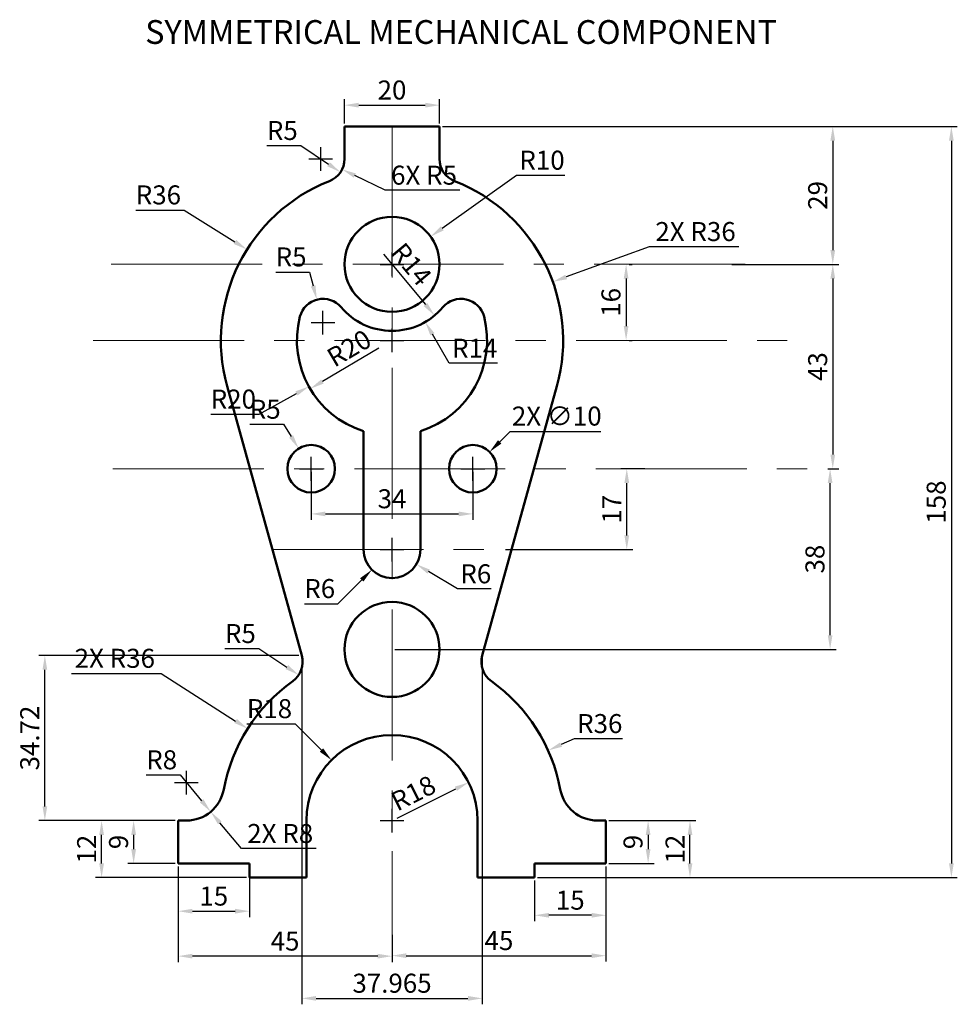
# Model space of a CAD drawing. Units: millimetres. Extents: x 53 to 250, y -7 to 201.
import ezdxf

# ---------------------------------------------------------------- set-up
doc = ezdxf.new("R2010")
doc.units = ezdxf.units.MM
doc.linetypes.add('CENTER', pattern=[50.8, 31.75, -6.35, 6.35, -6.35])
for name, color, linetype, lineweight in [('M-CNTR', 1, 'CENTER', 18), ('M-DIMS', 2, 'Continuous', 25), ('M-OUTL', 7, 'Continuous', 50), ('M-TEXT', 3, 'Continuous', 25)]:
    doc.layers.add(name, color=color, linetype=linetype, lineweight=lineweight)
doc.styles.get("Standard").update_dxf_attribs({"font": 'arial.ttf'})
doc.dimstyles.new('ISO-25', dxfattribs={"dimtxt": 4, "dimasz": 3, "dimexe": 1.25, "dimexo": 0.625, "dimtad": 1, "dimtoh": 1, "dimdec": 1, "dimtxsty": 'Standard', "dimcen": 2.5, "dimadec": 0, "dimazin": 0, "dimtfac": 1, "dimtdec": 1, "dimtofl": 0, "dimtmove": 0, "dimatfit": 3, "dimfxl": 1, "dimarcsym": 0})

# ---------------------------------------------------------------- blocks, each defined once
blk = doc.blocks.new('*D1')
at = {"layer": 'Defpoints', "color": 0, "transparency": 16777216}
for p in [(176.08, 32.09), (176.08, 23.09), (184.96, 23.09)]:
    blk.add_point(p, dxfattribs=at)
at = {"layer": 'M-DIMS', "color": 0, "lineweight": -2, "transparency": 16777216}
for p, q in [((176.7, 32.09), (186.21, 32.09)), ((184.96, 29.09), (184.96, 26.09)), ((176.7, 23.09), (186.21, 23.09))]:
    blk.add_line(p, q, dxfattribs=at)
at = {"layer": 'M-DIMS', "color": 0, "transparency": 16777216}
for points in [[(184.46, 29.09), (185.46, 29.09), (184.96, 32.09)], [(184.46, 26.09), (185.46, 26.09), (184.96, 23.09)]]:
    blk.add_solid(points, dxfattribs=at)
at = {"layer": 'M-DIMS', "color": 0, "transparency": 16777216, "insert": (182.3, 27.59), "char_height": 4, "attachment_point": 5, "rotation": 90}
blk.add_mtext('9', dxfattribs=at)
blk = doc.blocks.new('*D2')
at = {"layer": 'Defpoints', "color": 0, "transparency": 16777216}
for p in [(176.08, 32.09), (193.77, 32.09), (161.08, 20.09)]:
    blk.add_point(p, dxfattribs=at)
at = {"layer": 'M-DIMS', "color": 0, "lineweight": -2, "transparency": 16777216}
for p, q in [((176.7, 32.09), (195.02, 32.09)), ((193.77, 23.09), (193.77, 29.09)), ((161.7, 20.09), (195.02, 20.09))]:
    blk.add_line(p, q, dxfattribs=at)
at = {"layer": 'M-DIMS', "color": 0, "transparency": 16777216}
for points in [[(193.27, 29.09), (194.27, 29.09), (193.77, 32.09)], [(193.27, 23.09), (194.27, 23.09), (193.77, 20.09)]]:
    blk.add_solid(points, dxfattribs=at)
at = {"layer": 'M-DIMS', "color": 0, "transparency": 16777216, "insert": (191.14, 26.09), "char_height": 4, "attachment_point": 5, "rotation": 90}
blk.add_mtext('12', dxfattribs=at)
blk = doc.blocks.new('*D3')
at = {"layer": 'Defpoints', "color": 0, "transparency": 16777216}
for p in [(176.08, 23.09), (161.08, 20.09), (161.08, 12.18)]:
    blk.add_point(p, dxfattribs=at)
at = {"layer": 'M-DIMS', "color": 0, "lineweight": -2, "transparency": 16777216}
for p, q in [((176.08, 22.47), (176.08, 10.93)), ((161.08, 19.47), (161.08, 10.93)), ((173.08, 12.18), (164.08, 12.18))]:
    blk.add_line(p, q, dxfattribs=at)
at = {"layer": 'M-DIMS', "color": 0, "transparency": 16777216}
for points in [[(164.08, 12.68), (164.08, 11.68), (161.08, 12.18)], [(173.08, 12.68), (173.08, 11.68), (176.08, 12.18)]]:
    blk.add_solid(points, dxfattribs=at)
at = {"layer": 'M-DIMS', "color": 0, "transparency": 16777216, "insert": (168.58, 14.84), "char_height": 4, "attachment_point": 5}
blk.add_mtext('15', dxfattribs=at)
blk = doc.blocks.new('*D4')
at = {"layer": 'Defpoints', "color": 0, "transparency": 16777216}
for p in [(176.08, 23.09), (131.08, 7.05), (176.08, 3.68)]:
    blk.add_point(p, dxfattribs=at)
at = {"layer": 'M-DIMS', "color": 0, "lineweight": -2, "transparency": 16777216}
for p, q in [((176.08, 22.47), (176.08, 2.43)), ((131.08, 6.42), (131.08, 2.43)), ((134.08, 3.68), (173.08, 3.68))]:
    blk.add_line(p, q, dxfattribs=at)
at = {"layer": 'M-DIMS', "color": 0, "transparency": 16777216}
for points in [[(134.08, 4.18), (134.08, 3.18), (131.08, 3.68)], [(173.08, 4.18), (173.08, 3.18), (176.08, 3.68)]]:
    blk.add_solid(points, dxfattribs=at)
at = {"layer": 'M-DIMS', "color": 0, "transparency": 16777216, "insert": (153.58, 6.34), "char_height": 4, "attachment_point": 5}
blk.add_mtext('45', dxfattribs=at)
blk = doc.blocks.new('*D5')
at = {"layer": 'Defpoints', "color": 0, "transparency": 16777216}
for p in [(86.08, 23.09), (101.08, 23.09), (101.08, 13.04)]:
    blk.add_point(p, dxfattribs=at)
at = {"layer": 'M-DIMS', "color": 0, "lineweight": -2, "transparency": 16777216}
for p, q in [((86.08, 22.47), (86.08, 11.79)), ((101.08, 22.47), (101.08, 11.79)), ((89.08, 13.04), (98.08, 13.04))]:
    blk.add_line(p, q, dxfattribs=at)
at = {"layer": 'M-DIMS', "color": 0, "transparency": 16777216}
for points in [[(89.08, 13.54), (89.08, 12.54), (86.08, 13.04)], [(98.08, 13.54), (98.08, 12.54), (101.08, 13.04)]]:
    blk.add_solid(points, dxfattribs=at)
at = {"layer": 'M-DIMS', "color": 0, "transparency": 16777216, "insert": (93.58, 15.7), "char_height": 4, "attachment_point": 5}
blk.add_mtext('15', dxfattribs=at)
blk = doc.blocks.new('*D6')
at = {"layer": 'Defpoints', "color": 0, "transparency": 16777216}
for p in [(86.08, 32.09), (76.72, 23.09), (86.08, 23.09)]:
    blk.add_point(p, dxfattribs=at)
at = {"layer": 'M-DIMS', "color": 0, "lineweight": -2, "transparency": 16777216}
for p, q in [((85.45, 32.09), (75.47, 32.09)), ((76.72, 29.09), (76.72, 26.09)), ((85.45, 23.09), (75.47, 23.09))]:
    blk.add_line(p, q, dxfattribs=at)
at = {"layer": 'M-DIMS', "color": 0, "transparency": 16777216}
for points in [[(76.22, 29.09), (77.22, 29.09), (76.72, 32.09)], [(76.22, 26.09), (77.22, 26.09), (76.72, 23.09)]]:
    blk.add_solid(points, dxfattribs=at)
at = {"layer": 'M-DIMS', "color": 0, "transparency": 16777216, "insert": (74.06, 27.59), "char_height": 4, "attachment_point": 5, "rotation": 90}
blk.add_mtext('9', dxfattribs=at)
blk = doc.blocks.new('*D7')
at = {"layer": 'Defpoints', "color": 0, "transparency": 16777216}
for p in [(69.98, 32.09), (86.08, 32.09), (101.08, 20.09)]:
    blk.add_point(p, dxfattribs=at)
at = {"layer": 'M-DIMS', "color": 0, "lineweight": -2, "transparency": 16777216}
for p, q in [((85.45, 32.09), (68.73, 32.09)), ((69.98, 23.09), (69.98, 29.09)), ((100.45, 20.09), (68.73, 20.09))]:
    blk.add_line(p, q, dxfattribs=at)
at = {"layer": 'M-DIMS', "color": 0, "transparency": 16777216}
for points in [[(69.48, 29.09), (70.48, 29.09), (69.98, 32.09)], [(69.48, 23.09), (70.48, 23.09), (69.98, 20.09)]]:
    blk.add_solid(points, dxfattribs=at)
at = {"layer": 'M-DIMS', "color": 0, "transparency": 16777216, "insert": (67.35, 26.09), "char_height": 4, "attachment_point": 5, "rotation": 90}
blk.add_mtext('12', dxfattribs=at)
blk = doc.blocks.new('*D8')
at = {"layer": 'Defpoints', "color": 0, "transparency": 16777216}
for p in [(86.08, 23.09), (131.08, 8.69), (86.08, 3.58)]:
    blk.add_point(p, dxfattribs=at)
at = {"layer": 'M-DIMS', "color": 0, "lineweight": -2, "transparency": 16777216}
for p, q in [((86.08, 22.47), (86.08, 2.33)), ((131.08, 8.06), (131.08, 2.33)), ((128.08, 3.58), (89.08, 3.58))]:
    blk.add_line(p, q, dxfattribs=at)
at = {"layer": 'M-DIMS', "color": 0, "transparency": 16777216}
for points in [[(89.08, 4.08), (89.08, 3.08), (86.08, 3.58)], [(128.08, 4.08), (128.08, 3.08), (131.08, 3.58)]]:
    blk.add_solid(points, dxfattribs=at)
at = {"layer": 'M-DIMS', "color": 0, "transparency": 16777216, "insert": (108.58, 6.24), "char_height": 4, "attachment_point": 5}
blk.add_mtext('45', dxfattribs=at)
blk = doc.blocks.new('*D9')
at = {"layer": 'Defpoints', "color": 0, "transparency": 16777216}
for p in [(141.08, 178.09), (189.68, 20.09), (248.76, 20.09)]:
    blk.add_point(p, dxfattribs=at)
at = {"layer": 'M-DIMS', "color": 0, "lineweight": -2, "transparency": 16777216}
for p, q in [((141.7, 178.09), (250.01, 178.09)), ((248.76, 175.09), (248.76, 23.09)), ((190.31, 20.09), (250.01, 20.09))]:
    blk.add_line(p, q, dxfattribs=at)
at = {"layer": 'M-DIMS', "color": 0, "transparency": 16777216}
for points in [[(248.26, 175.09), (249.26, 175.09), (248.76, 178.09)], [(248.26, 23.09), (249.26, 23.09), (248.76, 20.09)]]:
    blk.add_solid(points, dxfattribs=at)
at = {"layer": 'M-DIMS', "color": 0, "transparency": 16777216, "insert": (246.09, 99.09), "char_height": 4, "attachment_point": 5, "rotation": 90}
blk.add_mtext('158', dxfattribs=at)
blk = doc.blocks.new('*D10')
at = {"layer": 'Defpoints', "color": 0, "transparency": 16777216}
for p in [(201.93, 178.09), (201.93, 149.09), (223.81, 149.09)]:
    blk.add_point(p, dxfattribs=at)
at = {"layer": 'M-DIMS', "color": 0, "lineweight": -2, "transparency": 16777216}
for p, q in [((202.55, 178.09), (225.06, 178.09)), ((223.81, 175.09), (223.81, 152.09)), ((202.55, 149.09), (225.06, 149.09))]:
    blk.add_line(p, q, dxfattribs=at)
at = {"layer": 'M-DIMS', "color": 0, "transparency": 16777216}
for points in [[(223.31, 175.09), (224.31, 175.09), (223.81, 178.09)], [(223.31, 152.09), (224.31, 152.09), (223.81, 149.09)]]:
    blk.add_solid(points, dxfattribs=at)
at = {"layer": 'M-DIMS', "color": 0, "transparency": 16777216, "insert": (221.15, 163.59), "char_height": 4, "attachment_point": 5, "rotation": 90}
blk.add_mtext('29', dxfattribs=at)
blk = doc.blocks.new('*D11')
at = {"layer": 'Defpoints', "color": 0, "transparency": 16777216}
for p in [(180.33, 149.09), (180.33, 133.09), (180.33, 133.09)]:
    blk.add_point(p, dxfattribs=at)
at = {"layer": 'M-DIMS', "color": 0, "lineweight": -2, "transparency": 16777216}
for p, q in [((180.95, 149.09), (181.58, 149.09)), ((180.33, 146.09), (180.33, 136.09)), ((180.95, 133.09), (181.58, 133.09))]:
    blk.add_line(p, q, dxfattribs=at)
at = {"layer": 'M-DIMS', "color": 0, "transparency": 16777216}
for points in [[(179.83, 146.09), (180.83, 146.09), (180.33, 149.09)], [(179.83, 136.09), (180.83, 136.09), (180.33, 133.09)]]:
    blk.add_solid(points, dxfattribs=at)
at = {"layer": 'M-DIMS', "color": 0, "transparency": 16777216, "insert": (177.66, 141.09), "char_height": 4, "attachment_point": 5, "rotation": 90}
blk.add_mtext('16', dxfattribs=at)
blk = doc.blocks.new('*D12')
at = {"layer": 'Defpoints', "color": 0, "transparency": 16777216}
for p in [(223.81, 149.09), (222.18, 106.09), (223.81, 106.09)]:
    blk.add_point(p, dxfattribs=at)
at = {"layer": 'M-DIMS', "color": 0, "lineweight": -2, "transparency": 16777216}
for p, q in [((224.44, 149.09), (225.06, 149.09)), ((223.81, 146.09), (223.81, 109.09)), ((222.8, 106.09), (225.06, 106.09))]:
    blk.add_line(p, q, dxfattribs=at)
at = {"layer": 'M-DIMS', "color": 0, "transparency": 16777216}
for points in [[(223.31, 146.09), (224.31, 146.09), (223.81, 149.09)], [(223.31, 109.09), (224.31, 109.09), (223.81, 106.09)]]:
    blk.add_solid(points, dxfattribs=at)
at = {"layer": 'M-DIMS', "color": 0, "transparency": 16777216, "insert": (221.15, 127.59), "char_height": 4, "attachment_point": 5, "rotation": 90}
blk.add_mtext('43', dxfattribs=at)
blk = doc.blocks.new('*D13')
at = {"layer": 'Defpoints', "color": 0, "transparency": 16777216}
for p in [(222.18, 106.09), (223.25, 106.09), (131.08, 68.09)]:
    blk.add_point(p, dxfattribs=at)
at = {"layer": 'M-DIMS', "color": 0, "lineweight": -2, "transparency": 16777216}
for p, q in [((222.8, 106.09), (224.5, 106.09)), ((223.25, 71.09), (223.25, 103.09)), ((131.7, 68.09), (224.5, 68.09))]:
    blk.add_line(p, q, dxfattribs=at)
at = {"layer": 'M-DIMS', "color": 0, "transparency": 16777216}
for points in [[(222.75, 103.09), (223.75, 103.09), (223.25, 106.09)], [(222.75, 71.09), (223.75, 71.09), (223.25, 68.09)]]:
    blk.add_solid(points, dxfattribs=at)
at = {"layer": 'M-DIMS', "color": 0, "transparency": 16777216, "insert": (220.58, 87.09), "char_height": 4, "attachment_point": 5, "rotation": 90}
blk.add_mtext('38', dxfattribs=at)
blk = doc.blocks.new('*D14')
at = {"layer": 'Defpoints', "color": 0, "transparency": 16777216}
for p in [(141.08, 182.57), (121.08, 178.09), (141.08, 178.09)]:
    blk.add_point(p, dxfattribs=at)
at = {"layer": 'M-DIMS', "color": 0, "lineweight": -2, "transparency": 16777216}
for p, q in [((121.08, 178.72), (121.08, 183.82)), ((124.08, 182.57), (138.08, 182.57)), ((141.08, 178.72), (141.08, 183.82))]:
    blk.add_line(p, q, dxfattribs=at)
at = {"layer": 'M-DIMS', "color": 0, "transparency": 16777216}
for points in [[(124.08, 183.07), (124.08, 182.07), (121.08, 182.57)], [(138.08, 183.07), (138.08, 182.07), (141.08, 182.57)]]:
    blk.add_solid(points, dxfattribs=at)
at = {"layer": 'M-DIMS', "color": 0, "transparency": 16777216, "insert": (131.08, 185.24), "char_height": 4, "attachment_point": 5}
blk.add_mtext('20', dxfattribs=at)
blk = doc.blocks.new('*D15')
at = {"layer": 'Defpoints', "color": 0, "transparency": 16777216}
for p in [(115.26, 141.68), (116.55, 136.84)]:
    blk.add_point(p, dxfattribs=at)
at = {"layer": 'M-DIMS', "color": 0, "lineweight": -2, "transparency": 16777216}
for p, q in [((106.61, 147.47), (113.71, 147.47)), ((113.71, 147.47), (114.49, 144.57)), ((116.55, 134.34), (116.55, 139.34)), ((114.05, 136.84), (119.05, 136.84))]:
    blk.add_line(p, q, dxfattribs=at)
at = {"layer": 'M-DIMS', "color": 0, "transparency": 16777216}
blk.add_solid([(114.97, 144.7), (114, 144.44), (115.26, 141.68)], dxfattribs=at)
at = {"layer": 'M-DIMS', "color": 0, "transparency": 16777216, "insert": (109.85, 150.13), "char_height": 4, "attachment_point": 5}
blk.add_mtext('R5', dxfattribs=at)
blk = doc.blocks.new('*D16')
at = {"layer": 'Defpoints', "color": 0, "transparency": 16777216}
for p in [(116.08, 171.25), (120.23, 168.47)]:
    blk.add_point(p, dxfattribs=at)
at = {"layer": 'M-DIMS', "color": 0, "lineweight": -2, "transparency": 16777216}
for p, q in [((104.76, 174.08), (111.87, 174.08)), ((111.87, 174.08), (117.74, 170.14))]:
    blk.add_line(p, q, dxfattribs=at)
at = {"layer": 'M-DIMS', "color": 0, "transparency": 16777216}
blk.add_solid([(118.02, 170.55), (117.46, 169.72), (120.23, 168.47)], dxfattribs=at)
at = {"layer": 'M-DIMS', "color": 0, "transparency": 16777216, "insert": (108, 176.73), "char_height": 4, "attachment_point": 5}
blk.add_mtext('R5', dxfattribs=at)
blk = doc.blocks.new('*D17')
at = {"layer": 'Defpoints', "color": 0, "transparency": 16777216}
for p in [(107.28, 65.48), (111.45, 62.73)]:
    blk.add_point(p, dxfattribs=at)
at = {"layer": 'M-DIMS', "color": 0, "lineweight": -2, "transparency": 16777216}
for p, q in [((95.94, 68.26), (103.04, 68.26)), ((103.04, 68.26), (108.95, 64.38))]:
    blk.add_line(p, q, dxfattribs=at)
at = {"layer": 'M-DIMS', "color": 0, "transparency": 16777216}
blk.add_solid([(109.22, 64.8), (108.67, 63.96), (111.45, 62.73)], dxfattribs=at)
at = {"layer": 'M-DIMS', "color": 0, "transparency": 16777216, "insert": (99.18, 70.92), "char_height": 4, "attachment_point": 5}
blk.add_mtext('R5', dxfattribs=at)
blk = doc.blocks.new('*D18')
at = {"layer": 'Defpoints', "color": 0, "transparency": 16777216}
for p in [(114.08, 106.09), (148.08, 106.09), (148.08, 96.6)]:
    blk.add_point(p, dxfattribs=at)
at = {"layer": 'M-DIMS', "color": 0, "lineweight": -2, "transparency": 16777216}
for p, q in [((114.08, 105.47), (114.08, 95.35)), ((148.08, 105.47), (148.08, 95.35)), ((117.08, 96.6), (145.08, 96.6))]:
    blk.add_line(p, q, dxfattribs=at)
at = {"layer": 'M-DIMS', "color": 0, "transparency": 16777216}
for points in [[(117.08, 97.1), (117.08, 96.1), (114.08, 96.6)], [(145.08, 97.1), (145.08, 96.1), (148.08, 96.6)]]:
    blk.add_solid(points, dxfattribs=at)
at = {"layer": 'M-DIMS', "color": 0, "transparency": 16777216, "insert": (131.08, 99.27), "char_height": 4, "attachment_point": 5}
blk.add_mtext('34', dxfattribs=at)
blk = doc.blocks.new('*D19')
at = {"layer": 'Defpoints', "color": 0, "transparency": 16777216}
for p in [(131.08, 89.09), (136.22, 86)]:
    blk.add_point(p, dxfattribs=at)
at = {"layer": 'M-DIMS', "color": 0, "lineweight": -2, "transparency": 16777216}
for p, q in [((131.08, 86.59), (131.08, 91.59)), ((128.58, 89.09), (133.58, 89.09)), ((144.86, 80.81), (138.79, 84.46)), ((151.94, 80.81), (144.86, 80.81))]:
    blk.add_line(p, q, dxfattribs=at)
at = {"layer": 'M-DIMS', "color": 0, "transparency": 16777216}
blk.add_solid([(139.05, 84.89), (138.53, 84.03), (136.22, 86)], dxfattribs=at)
at = {"layer": 'M-DIMS', "color": 0, "transparency": 16777216, "insert": (148.71, 83.48), "char_height": 4, "attachment_point": 5}
blk.add_mtext('R6', dxfattribs=at)
blk = doc.blocks.new('*D20')
at = {"layer": 'Defpoints', "color": 0, "transparency": 16777216}
for p in [(139.21, 154.91), (131.08, 149.09)]:
    blk.add_point(p, dxfattribs=at)
at = {"layer": 'M-DIMS', "color": 0, "lineweight": -2, "transparency": 16777216}
for p, q in [((157.24, 167.81), (141.65, 156.66)), ((167.41, 167.81), (157.24, 167.81)), ((131.08, 146.59), (131.08, 151.59)), ((128.58, 149.09), (133.58, 149.09))]:
    blk.add_line(p, q, dxfattribs=at)
at = {"layer": 'M-DIMS', "color": 0, "transparency": 16777216}
blk.add_solid([(141.36, 157.07), (141.94, 156.25), (139.21, 154.91)], dxfattribs=at)
at = {"layer": 'M-DIMS', "color": 0, "transparency": 16777216, "insert": (162.64, 170.48), "char_height": 4, "attachment_point": 5}
blk.add_mtext('R10', dxfattribs=at)
blk = doc.blocks.new('*D21')
at = {"layer": 'Defpoints', "color": 0, "transparency": 16777216}
for p in [(131.08, 133.09), (113.86, 122.92)]:
    blk.add_point(p, dxfattribs=at)
at = {"layer": 'M-DIMS', "color": 0, "lineweight": -2, "transparency": 16777216}
blk.add_line((128.32, 131.46), (116.44, 124.45), dxfattribs=at)
at = {"layer": 'M-DIMS', "color": 0, "transparency": 16777216}
blk.add_solid([(116.19, 124.88), (116.7, 124.01), (113.86, 122.92)], dxfattribs=at)
at = {"layer": 'M-DIMS', "color": 0, "transparency": 16777216, "insert": (122.31, 131.01), "char_height": 4, "attachment_point": 5, "rotation": 30.5845}
blk.add_mtext('R20', dxfattribs=at)
blk = doc.blocks.new('*D22')
at = {"layer": 'Defpoints', "color": 0, "transparency": 16777216}
for p in [(131.08, 149.09), (140.04, 138.34)]:
    blk.add_point(p, dxfattribs=at)
at = {"layer": 'M-DIMS', "color": 0, "lineweight": -2, "transparency": 16777216}
blk.add_line((129.29, 151.24), (138.12, 140.64), dxfattribs=at)
at = {"layer": 'M-DIMS', "color": 0, "transparency": 16777216}
blk.add_solid([(138.5, 140.96), (137.73, 140.32), (140.04, 138.34)], dxfattribs=at)
at = {"layer": 'M-DIMS', "color": 0, "transparency": 16777216, "insert": (134.77, 148.78), "char_height": 4, "attachment_point": 5, "rotation": 309.7865}
blk.add_mtext('R14', dxfattribs=at)
blk = doc.blocks.new('*D23')
at = {"layer": 'Defpoints', "color": 0, "transparency": 16777216}
for p in [(100.57, 152.21), (131.08, 133.09)]:
    blk.add_point(p, dxfattribs=at)
at = {"layer": 'M-DIMS', "color": 0, "lineweight": -2, "transparency": 16777216}
for p, q in [((77.15, 160.51), (87.33, 160.51)), ((87.33, 160.51), (98.03, 153.81)), ((131.08, 130.59), (131.08, 135.59)), ((128.58, 133.09), (133.58, 133.09))]:
    blk.add_line(p, q, dxfattribs=at)
at = {"layer": 'M-DIMS', "color": 0, "transparency": 16777216}
blk.add_solid([(98.3, 154.23), (97.77, 153.38), (100.57, 152.21)], dxfattribs=at)
at = {"layer": 'M-DIMS', "color": 0, "transparency": 16777216, "insert": (81.93, 163.18), "char_height": 4, "attachment_point": 5}
blk.add_mtext('R36', dxfattribs=at)
blk = doc.blocks.new('*D24')
at = {"layer": 'Defpoints', "color": 0, "transparency": 16777216}
for p in [(180.47, 106.09), (184.9, 106.09), (154.32, 89.09)]:
    blk.add_point(p, dxfattribs=at)
at = {"layer": 'M-DIMS', "color": 0, "lineweight": -2, "transparency": 16777216}
for p, q in [((184.27, 106.09), (179.22, 106.09)), ((180.47, 92.09), (180.47, 103.09)), ((154.95, 89.09), (181.72, 89.09))]:
    blk.add_line(p, q, dxfattribs=at)
at = {"layer": 'M-DIMS', "color": 0, "transparency": 16777216}
for points in [[(179.97, 103.09), (180.97, 103.09), (180.47, 106.09)], [(179.97, 92.09), (180.97, 92.09), (180.47, 89.09)]]:
    blk.add_solid(points, dxfattribs=at)
at = {"layer": 'M-DIMS', "color": 0, "transparency": 16777216, "insert": (177.84, 97.59), "char_height": 4, "attachment_point": 5, "rotation": 90}
blk.add_mtext('17', dxfattribs=at)
blk = doc.blocks.new('*D25')
at = {"layer": 'Defpoints', "color": 0, "transparency": 16777216}
for p in [(111.44, 110.34), (114.08, 106.09)]:
    blk.add_point(p, dxfattribs=at)
at = {"layer": 'M-DIMS', "color": 0, "lineweight": -2, "transparency": 16777216}
for p, q in [((101.17, 115.44), (108.27, 115.44)), ((108.27, 115.44), (109.85, 112.89)), ((114.08, 103.59), (114.08, 108.59)), ((111.58, 106.09), (116.58, 106.09))]:
    blk.add_line(p, q, dxfattribs=at)
at = {"layer": 'M-DIMS', "color": 0, "transparency": 16777216}
blk.add_solid([(110.28, 113.15), (109.43, 112.63), (111.44, 110.34)], dxfattribs=at)
at = {"layer": 'M-DIMS', "color": 0, "transparency": 16777216, "insert": (104.41, 118.1), "char_height": 4, "attachment_point": 5}
blk.add_mtext('R5', dxfattribs=at)
blk = doc.blocks.new('*D26')
at = {"layer": 'Defpoints', "color": 0, "transparency": 16777216}
for p in [(147.19, 40.12), (131.08, 32.09)]:
    blk.add_point(p, dxfattribs=at)
at = {"layer": 'M-DIMS', "color": 0, "lineweight": -2, "transparency": 16777216}
blk.add_line((132.14, 32.62), (144.5, 38.78), dxfattribs=at)
at = {"layer": 'M-DIMS', "color": 0, "transparency": 16777216}
blk.add_solid([(144.28, 39.23), (144.73, 38.34), (147.19, 40.12)], dxfattribs=at)
at = {"layer": 'M-DIMS', "color": 0, "transparency": 16777216, "insert": (135.79, 37.42), "char_height": 4, "attachment_point": 5, "rotation": 26.4797}
blk.add_mtext('R18', dxfattribs=at)
blk = doc.blocks.new('*D27')
at = {"layer": 'Defpoints', "color": 0, "transparency": 16777216}
for p in [(163.92, 46.85), (131.08, 32.09)]:
    blk.add_point(p, dxfattribs=at)
at = {"layer": 'M-DIMS', "color": 0, "lineweight": -2, "transparency": 16777216}
for p, q in [((169.39, 49.31), (166.65, 48.08)), ((179.57, 49.31), (169.39, 49.31)), ((131.08, 29.59), (131.08, 34.59)), ((128.58, 32.09), (133.58, 32.09))]:
    blk.add_line(p, q, dxfattribs=at)
at = {"layer": 'M-DIMS', "color": 0, "transparency": 16777216}
blk.add_solid([(166.45, 48.53), (166.86, 47.62), (163.92, 46.85)], dxfattribs=at)
at = {"layer": 'M-DIMS', "color": 0, "transparency": 16777216, "insert": (174.79, 51.98), "char_height": 4, "attachment_point": 5}
blk.add_mtext('R36', dxfattribs=at)
blk = doc.blocks.new('*D28')
at = {"layer": 'Defpoints', "color": 0, "transparency": 16777216}
for p in [(87.81, 40.09), (92.93, 33.95)]:
    blk.add_point(p, dxfattribs=at)
at = {"layer": 'M-DIMS', "color": 0, "lineweight": -2, "transparency": 16777216}
for p, q in [((79.39, 41.7), (86.48, 41.7)), ((86.48, 41.7), (91.01, 36.26))]:
    blk.add_line(p, q, dxfattribs=at)
at = {"layer": 'M-DIMS', "color": 0, "transparency": 16777216}
blk.add_solid([(91.4, 36.58), (90.63, 35.93), (92.93, 33.95)], dxfattribs=at)
at = {"layer": 'M-DIMS', "color": 0, "transparency": 16777216, "insert": (82.62, 44.36), "char_height": 4, "attachment_point": 5}
blk.add_mtext('R8', dxfattribs=at)
blk = doc.blocks.new('*D29')
at = {"layer": 'Defpoints', "color": 0, "transparency": 16777216}
for p in [(112.1, 66.82), (150.06, 66.82), (150.06, -5.3)]:
    blk.add_point(p, dxfattribs=at)
at = {"layer": 'M-DIMS', "color": 0, "lineweight": -2, "transparency": 16777216}
for p, q in [((112.1, 66.19), (112.1, -6.55)), ((150.06, 66.19), (150.06, -6.55)), ((115.1, -5.3), (147.06, -5.3))]:
    blk.add_line(p, q, dxfattribs=at)
at = {"layer": 'M-DIMS', "color": 0, "transparency": 16777216}
for points in [[(115.1, -4.8), (115.1, -5.8), (112.1, -5.3)], [(147.06, -4.8), (147.06, -5.8), (150.06, -5.3)]]:
    blk.add_solid(points, dxfattribs=at)
at = {"layer": 'M-DIMS', "color": 0, "transparency": 16777216, "insert": (131.08, -2.63), "char_height": 4, "attachment_point": 5}
blk.add_mtext('37.965', dxfattribs=at)
blk = doc.blocks.new('*D30')
at = {"layer": 'Defpoints', "color": 0, "transparency": 16777216}
for p in [(58.04, 66.82), (112.1, 66.82), (86.08, 32.09)]:
    blk.add_point(p, dxfattribs=at)
at = {"layer": 'M-DIMS', "color": 0, "lineweight": -2, "transparency": 16777216}
for p, q in [((111.47, 66.82), (56.79, 66.82)), ((58.04, 35.09), (58.04, 63.82)), ((85.45, 32.09), (56.79, 32.09))]:
    blk.add_line(p, q, dxfattribs=at)
at = {"layer": 'M-DIMS', "color": 0, "transparency": 16777216}
for points in [[(57.54, 63.82), (58.54, 63.82), (58.04, 66.82)], [(57.54, 35.09), (58.54, 35.09), (58.04, 32.09)]]:
    blk.add_solid(points, dxfattribs=at)
at = {"layer": 'M-DIMS', "color": 0, "transparency": 16777216, "insert": (55.37, 49.46), "char_height": 4, "attachment_point": 5, "rotation": 90}
blk.add_mtext('34.72', dxfattribs=at)
blk = doc.blocks.new('*D31')
at = {"layer": 'Defpoints', "color": 0, "transparency": 16777216}
for p in [(164.91, 145.41), (131.08, 133.09)]:
    blk.add_point(p, dxfattribs=at)
at = {"layer": 'M-DIMS', "color": 0, "lineweight": -2, "transparency": 16777216}
for p, q in [((185.2, 152.8), (167.73, 146.43)), ((204.05, 152.8), (185.2, 152.8)), ((131.08, 130.59), (131.08, 135.59)), ((128.58, 133.09), (133.58, 133.09))]:
    blk.add_line(p, q, dxfattribs=at)
at = {"layer": 'M-DIMS', "color": 0, "transparency": 16777216}
blk.add_solid([(167.55, 146.9), (167.9, 145.96), (164.91, 145.41)], dxfattribs=at)
at = {"layer": 'M-DIMS', "color": 0, "transparency": 16777216, "insert": (194.94, 155.47), "char_height": 4, "attachment_point": 5}
blk.add_mtext('2X R36', dxfattribs=at)
blk = doc.blocks.new('*D32')
at = {"layer": 'Defpoints', "color": 0, "transparency": 16777216}
for p in [(100.71, 51.43), (131.08, 32.09)]:
    blk.add_point(p, dxfattribs=at)
at = {"layer": 'M-DIMS', "color": 0, "lineweight": -2, "transparency": 16777216}
for p, q in [((63.65, 63.04), (82.49, 63.04)), ((82.49, 63.04), (98.18, 53.04)), ((131.08, 29.59), (131.08, 34.59)), ((128.58, 32.09), (133.58, 32.09))]:
    blk.add_line(p, q, dxfattribs=at)
at = {"layer": 'M-DIMS', "color": 0, "transparency": 16777216}
blk.add_solid([(98.45, 53.47), (97.91, 52.62), (100.71, 51.43)], dxfattribs=at)
at = {"layer": 'M-DIMS', "color": 0, "transparency": 16777216, "insert": (72.76, 65.71), "char_height": 4, "attachment_point": 5}
blk.add_mtext('2X R36', dxfattribs=at)
blk = doc.blocks.new('*D33')
at = {"layer": 'Defpoints', "color": 0, "transparency": 16777216}
for p in [(131.08, 133.09), (113.59, 123.39)]:
    blk.add_point(p, dxfattribs=at)
at = {"layer": 'M-DIMS', "color": 0, "lineweight": -2, "transparency": 16777216}
for p, q in [((131.08, 130.59), (131.08, 135.59)), ((128.58, 133.09), (133.58, 133.09)), ((103.1, 117.57), (110.97, 121.93)), ((92.93, 117.57), (103.1, 117.57))]:
    blk.add_line(p, q, dxfattribs=at)
at = {"layer": 'M-DIMS', "color": 0, "transparency": 16777216}
blk.add_solid([(110.72, 122.37), (111.21, 121.5), (113.59, 123.39)], dxfattribs=at)
at = {"layer": 'M-DIMS', "color": 0, "transparency": 16777216, "insert": (97.7, 120.23), "char_height": 4, "attachment_point": 5}
blk.add_mtext('R20', dxfattribs=at)
blk = doc.blocks.new('*D34')
at = {"layer": 'Defpoints', "color": 0, "transparency": 16777216}
for p in [(118.35, 44.82), (131.08, 32.09)]:
    blk.add_point(p, dxfattribs=at)
at = {"layer": 'M-DIMS', "color": 0, "lineweight": -2, "transparency": 16777216}
for p, q in [((100.52, 52.46), (110.71, 52.46)), ((110.71, 52.46), (116.23, 46.94)), ((131.08, 29.59), (131.08, 34.59)), ((128.58, 32.09), (133.58, 32.09))]:
    blk.add_line(p, q, dxfattribs=at)
at = {"layer": 'M-DIMS', "color": 0, "transparency": 16777216}
blk.add_solid([(116.58, 47.3), (115.87, 46.59), (118.35, 44.82)], dxfattribs=at)
at = {"layer": 'M-DIMS', "color": 0, "transparency": 16777216, "insert": (105.3, 55.12), "char_height": 4, "attachment_point": 5}
blk.add_mtext('R18', dxfattribs=at)
blk = doc.blocks.new('*D35')
at = {"layer": 'Defpoints', "color": 0, "transparency": 16777216}
for p in [(131.08, 149.09), (138.08, 136.97)]:
    blk.add_point(p, dxfattribs=at)
at = {"layer": 'M-DIMS', "color": 0, "lineweight": -2, "transparency": 16777216}
for p, q in [((131.08, 146.59), (131.08, 151.59)), ((128.58, 149.09), (133.58, 149.09)), ((143.09, 128.3), (139.58, 134.37)), ((153.26, 128.3), (143.09, 128.3))]:
    blk.add_line(p, q, dxfattribs=at)
at = {"layer": 'M-DIMS', "color": 0, "transparency": 16777216}
blk.add_solid([(140.01, 134.62), (139.15, 134.12), (138.08, 136.97)], dxfattribs=at)
at = {"layer": 'M-DIMS', "color": 0, "transparency": 16777216, "insert": (148.48, 130.93), "char_height": 4, "attachment_point": 5}
blk.add_mtext('R14', dxfattribs=at)
blk = doc.blocks.new('*D36')
at = {"layer": 'Defpoints', "color": 0, "transparency": 16777216}
for p in [(87.81, 40.09), (92.93, 33.95)]:
    blk.add_point(p, dxfattribs=at)
at = {"layer": 'M-DIMS', "color": 0, "lineweight": -2, "transparency": 16777216}
for p, q in [((87.81, 37.59), (87.81, 42.59)), ((85.31, 40.09), (90.31, 40.09)), ((99.38, 26.19), (94.85, 31.64)), ((115.12, 26.19), (99.38, 26.19))]:
    blk.add_line(p, q, dxfattribs=at)
at = {"layer": 'M-DIMS', "color": 0, "transparency": 16777216}
blk.add_solid([(95.23, 31.96), (94.46, 31.32), (92.93, 33.95)], dxfattribs=at)
at = {"layer": 'M-DIMS', "color": 0, "transparency": 16777216, "insert": (107.56, 28.86), "char_height": 4, "attachment_point": 5}
blk.add_mtext('2X R8', dxfattribs=at)
blk = doc.blocks.new('*D37')
at = {"layer": 'Defpoints', "color": 0, "transparency": 16777216}
for p in [(131.08, 89.09), (126.84, 84.85)]:
    blk.add_point(p, dxfattribs=at)
at = {"layer": 'M-DIMS', "color": 0, "lineweight": -2, "transparency": 16777216}
for p, q in [((131.08, 86.59), (131.08, 91.59)), ((128.58, 89.09), (133.58, 89.09)), ((119.71, 77.71), (124.72, 82.73)), ((112.64, 77.71), (119.71, 77.71))]:
    blk.add_line(p, q, dxfattribs=at)
at = {"layer": 'M-DIMS', "color": 0, "transparency": 16777216}
blk.add_solid([(124.37, 83.08), (125.07, 82.37), (126.84, 84.85)], dxfattribs=at)
at = {"layer": 'M-DIMS', "color": 0, "transparency": 16777216, "insert": (115.87, 80.38), "char_height": 4, "attachment_point": 5}
blk.add_mtext('R6', dxfattribs=at)
blk = doc.blocks.new('*D38')
at = {"layer": 'Defpoints', "color": 0, "transparency": 16777216}
for p in [(116.08, 171.25), (120.57, 169.07)]:
    blk.add_point(p, dxfattribs=at)
at = {"layer": 'M-DIMS', "color": 0, "lineweight": -2, "transparency": 16777216}
for p, q in [((116.08, 168.75), (116.08, 173.75)), ((113.58, 171.25), (118.58, 171.25)), ((129.64, 164.66), (123.27, 167.76)), ((145.37, 164.66), (129.64, 164.66))]:
    blk.add_line(p, q, dxfattribs=at)
at = {"layer": 'M-DIMS', "color": 0, "transparency": 16777216}
blk.add_solid([(123.49, 168.2), (123.05, 167.31), (120.57, 169.07)], dxfattribs=at)
at = {"layer": 'M-DIMS', "color": 0, "transparency": 16777216, "insert": (137.82, 167.33), "char_height": 4, "attachment_point": 5}
blk.add_mtext('6X R5', dxfattribs=at)
blk = doc.blocks.new('*D39')
at = {"layer": 'Defpoints', "color": 0, "transparency": 16777216}
for p in [(151.61, 109.63), (144.54, 102.56)]:
    blk.add_point(p, dxfattribs=at)
at = {"layer": 'M-DIMS', "color": 0, "lineweight": -2, "transparency": 16777216}
for p, q in [((155.85, 113.88), (153.73, 111.75)), ((175, 113.88), (155.85, 113.88)), ((148.08, 103.59), (148.08, 108.59)), ((145.58, 106.09), (150.58, 106.09))]:
    blk.add_line(p, q, dxfattribs=at)
at = {"layer": 'M-DIMS', "color": 0, "transparency": 16777216}
blk.add_solid([(153.38, 112.11), (154.09, 111.4), (151.61, 109.63)], dxfattribs=at)
at = {"layer": 'M-DIMS', "color": 0, "transparency": 16777216, "insert": (165.74, 116.66), "char_height": 4, "attachment_point": 5}
blk.add_mtext('2X ∅10', dxfattribs=at)

msp = doc.modelspace()

# ---------------------------------------------------------------- linework, layer by layer
at = {"layer": 'M-CNTR'}
for p, q in [((131.0775, 178.0949), (131.0775, 4.8529)), ((72.0093, 149.0949), (206.1978, 149.0949)), ((68.189, 133.0949), (218.1545, 133.0949)), ((72.3685, 106.0949), (222.1783, 106.0949)), ((105.9182, 89.0949), (156.2367, 89.0949))]:
    msp.add_line(p, q, dxfattribs=at)
at = {"layer": 'M-OUTL'}
for p, q in [((121.0775, 178.0949), (141.0775, 178.0949)), ((121.0775, 178.0949), (121.0775, 171.2525)), ((141.0775, 178.0949), (141.0775, 171.2525)), ((96.386, 123.477), (112.0951, 66.8153)), ((165.7689, 123.477), (150.0599, 66.8153)), ((125.0775, 89.0949), (125.0775, 114.0161)), ((137.0775, 89.0949), (137.0775, 114.0161)), ((87.8108, 32.0949), (86.0775, 32.0949)), ((86.0775, 32.0949), (86.0775, 23.0949)), ((113.0775, 20.0949), (113.0775, 32.0949)), ((149.0775, 32.0949), (149.0775, 20.0949)), ((174.3441, 32.0949), (176.0775, 32.0949)), ((176.0775, 32.0949), (176.0775, 23.0949)), ((86.0775, 23.0949), (101.0775, 23.0949)), ((101.0775, 23.0949), (101.0775, 20.0949)), ((176.0775, 23.0949), (161.0775, 23.0949)), ((161.0775, 23.0949), (161.0775, 20.0949)), ((101.0775, 20.0949), (113.0775, 20.0949)), ((149.0775, 20.0949), (161.0775, 20.0949))]:
    msp.add_line(p, q, dxfattribs=at)
for centre, radius in [((131.0775, 149.0949), 10), ((114.0775, 106.0949), 5), ((148.0775, 106.0949), 5), ((131.0775, 68.0949), 10)]:
    msp.add_circle(centre, radius, dxfattribs=at)
for centre, radius, start, end in [((116.0775, 171.2525), 5, 291.460128, 0), ((146.0775, 171.2525), 5, 180, 248.539872), ((131.0775, 133.0949), 36, 111.460128, 195.495638), ((131.0775, 133.0949), 36, 344.504362, 68.539872), ((116.5538, 136.8449), 5, 40.145948, 165.522488), ((145.6011, 136.8449), 5, 14.477512, 139.854052), ((131.0775, 149.0949), 14, 220.145948, 319.854052), ((131.0775, 133.0949), 20, 165.522488, 252.542397), ((131.0775, 133.0949), 20, 287.457603, 14.477512), ((131.0775, 89.0949), 6, 180, 360), ((107.2768, 65.4795), 5, 305.485983, 15.495638), ((154.8781, 65.4795), 5, 164.504362, 234.514017), ((131.0775, 32.0949), 36, 125.485983, 169.524318), ((131.0775, 32.0949), 36, 10.475682, 54.514017), ((131.0775, 32.0949), 18, 0, 180), ((87.8108, 40.0949), 8, 270, 349.524318), ((174.3441, 40.0949), 8, 190.475682, 270)]:
    msp.add_arc(centre, radius, start, end, dxfattribs=at)

# ---------------------------------------------------------------- texts
at = {"layer": 'M-TEXT', "insert": (79.147, 200.4589), "char_height": 5, "attachment_point": 1}
msp.add_mtext_dynamic_manual_height_columns('SYMMETRICAL MECHANICAL COMPONENT', width=149.805564, gutter_width=12.5, heights=[0], dxfattribs=at)

# ---------------------------------------------------------------- dimensions: what is measured, and where the dimension line sits
at = {"layer": 'M-DIMS'}
for base, p1, p2, override, picture, middle in [((141.0775, 182.5704), (121.0775, 178.0949), (141.0775, 178.0949), {"dimclrd": 0, "dimclre": 0, "dimclrt": 0}, '*D14', (131.0775, 185.2377)), ((148.0775, 96.5992), (114.0775, 106.0949), (148.0775, 106.0949), {"dimclrd": 0, "dimclre": 0, "dimclrt": 0}, '*D18', (131.0775, 99.2679)), ((150.0599, -5.2971), (112.0951, 66.8153), (150.0599, 66.8153), {"dimdec": 3, "dimlfac": 1, "dimrnd": 0, "dimzin": 0, "dimdsep": 46, "dimlunit": 2}, '*D29', (131.0775, -2.6285)), ((101.0775, 13.0351), (86.0775, 23.0949), (101.0775, 23.0949), {"dimclrd": 0, "dimclre": 0, "dimclrt": 0}, '*D5', (93.5775, 15.7024)), ((86.0775, 3.5815), (131.0775, 8.6886), (86.0775, 23.0949), {"dimclrd": 0, "dimclre": 0, "dimclrt": 0}, '*D8', (108.5775, 6.2406)), ((176.0775, 3.6794), (131.0775, 7.0479), (176.0775, 23.0949), {"dimclrd": 0, "dimclre": 0, "dimclrt": 0}, '*D4', (153.5775, 6.3385)), ((161.0775, 12.1767), (176.0775, 23.0949), (161.0775, 20.0949), {"dimclrd": 0, "dimclre": 0, "dimclrt": 0}, '*D3', (168.5775, 14.844))]:
    dim = msp.add_linear_dim(base=base, p1=p1, p2=p2, dimstyle='ISO-25', override=override, dxfattribs=at)
    dim.commit()
    dim.dimension.update_dxf_attribs({"geometry": picture, "text_midpoint": middle})
for center, mpoint, override, picture, middle in [((116.0775, 171.2525), (120.23, 168.4674), {"dimclrd": 0, "dimclre": 0, "dimclrt": 0}, '*D16', (108.0032, 174.0755)), ((131.0775, 149.0949), (139.2105, 154.9133), {"dimclrd": 0, "dimclre": 0, "dimclrt": 0}, '*D20', (162.6387, 167.8129)), ((131.0775, 133.0949), (100.5744, 152.2146), {"dimclrd": 0, "dimclre": 0, "dimclrt": 0}, '*D23', (81.931, 160.514)), ((131.0775, 149.0949), (140.0365, 138.3368), {"dimclrd": 0, "dimclre": 0, "dimclrt": 0}, '*D22', (132.744, 147.0938)), ((131.0775, 133.0949), (113.5906, 123.3888), {"dimdec": 0, "dimlfac": 1, "dimrnd": 0, "dimzin": 0, "dimdsep": 46, "dimlunit": 2}, '*D33', (97.7013, 117.5651)), ((131.0775, 133.0949), (113.8599, 122.9187), {"dimclrd": 0, "dimclre": 0, "dimclrt": 0}, '*D21', (123.6715, 128.7177)), ((107.2768, 65.4795), (111.4544, 62.7321), {"dimclrd": 0, "dimclre": 0, "dimclrt": 0}, '*D17', (99.1771, 68.2643)), ((131.0775, 32.0949), (118.3484, 44.8216), {"dimdec": 0, "dimlfac": 1, "dimrnd": 0, "dimzin": 0, "dimdsep": 46, "dimlunit": 2}, '*D34', (105.3028, 52.4577)), ((87.8108, 40.0949), (92.9349, 33.9513), {"dimclrd": 0, "dimclre": 0, "dimclrt": 0}, '*D28', (82.6215, 41.6958)), ((131.0775, 32.0949), (147.1891, 40.1208), {"dimclrd": 0, "dimclre": 0, "dimclrt": 0}, '*D26', (136.9778, 35.0341))]:
    dim = msp.add_radius_dim(center=center, mpoint=mpoint, dimstyle='ISO-25', override=override, dxfattribs=at)
    dim.commit()
    dim.dimension.update_dxf_attribs({"geometry": picture, "text_midpoint": middle, "dimtype": 164})
for base, p1, p2, override, picture, middle in [((248.7613, 20.0949), (141.0775, 178.0949), (189.6834, 20.0949), {"dimclrd": 0, "dimclre": 0, "dimclrt": 0}, '*D9', (246.094, 99.0949)), ((223.8142, 149.0949), (201.9281, 178.0949), (201.9281, 149.0949), {"dimclrd": 0, "dimclre": 0, "dimclrt": 0}, '*D10', (221.1469, 163.5949)), ((180.3262, 133.0949), (180.3262, 149.0949), (180.3262, 133.0949), {"dimclrd": 0, "dimclre": 0, "dimclrt": 0}, '*D11', (177.6589, 141.0949)), ((223.8142, 106.0949), (223.8142, 149.0949), (222.1783, 106.0949), {"dimclrd": 0, "dimclre": 0, "dimclrt": 0}, '*D12', (221.1455, 127.5949)), ((223.2457, 106.0949), (131.0775, 68.0949), (222.1783, 106.0949), {"dimclrd": 0, "dimclre": 0, "dimclrt": 0}, '*D13', (220.5771, 87.0949)), ((180.4711, 106.0949), (154.3242, 89.0949), (184.8992, 106.0949), {"dimclrd": 0, "dimclre": 0, "dimclrt": 0}, '*D24', (177.8379, 97.5949)), ((58.039, 66.8153), (86.0775, 32.0949), (112.0951, 66.8153), {"dimdec": 2, "dimlfac": 1, "dimrnd": 0, "dimzin": 0, "dimdsep": 46, "dimlunit": 2}, '*D30', (55.3704, 49.4551)), ((69.9801, 32.0949), (101.0775, 20.0949), (86.0775, 32.0949), {"dimclrd": 0, "dimclre": 0, "dimclrt": 0}, '*D7', (67.3469, 26.0949)), ((76.723, 23.0949), (86.0775, 32.0949), (86.0775, 23.0949), {"dimclrd": 0, "dimclre": 0, "dimclrt": 0}, '*D6', (74.0557, 27.5949)), ((193.7717, 32.0949), (161.0775, 20.0949), (176.0775, 32.0949), {"dimclrd": 0, "dimclre": 0, "dimclrt": 0}, '*D2', (191.1385, 26.0949)), ((184.9624, 23.0949), (176.0775, 32.0949), (176.0775, 23.0949), {"dimclrd": 0, "dimclre": 0, "dimclrt": 0}, '*D1', (182.2951, 27.5949))]:
    dim = msp.add_linear_dim(base=base, p1=p1, p2=p2, angle=90, dimstyle='ISO-25', override=override, dxfattribs=at)
    dim.commit()
    dim.dimension.update_dxf_attribs({"geometry": picture, "text_midpoint": middle})
for center, mpoint, text, picture, middle in [((116.0775, 171.2525), (120.5744, 169.0666), '6X <>', '*D38', (137.8177, 167.3253)), ((87.8108, 40.0949), (92.9277, 33.9453), '2X <>', '*D36', (107.5637, 28.8606))]:
    dim = msp.add_radius_dim(center=center, mpoint=mpoint, text=text, dimstyle='ISO-25', override={"dimdec": 0, "dimlfac": 1, "dimrnd": 0, "dimzin": 0, "dimdsep": 46, "dimlunit": 2}, dxfattribs=at)
    dim.commit()
    dim.dimension.update_dxf_attribs({"geometry": picture, "text_midpoint": middle})
for center, mpoint, picture, middle in [((131.0775, 133.0949), (164.9061, 145.4086), '*D31', (194.9374, 152.7968)), ((131.0775, 32.0949), (100.7126, 51.4333), '*D32', (72.7595, 63.0364))]:
    dim = msp.add_radius_dim(center=center, mpoint=mpoint, text='2X <>', dimstyle='ISO-25', override={"dimdec": 0, "dimlfac": 1, "dimrnd": 0, "dimzin": 0, "dimdsep": 46, "dimlunit": 2}, dxfattribs=at)
    dim.commit()
    dim.dimension.update_dxf_attribs({"geometry": picture, "text_midpoint": middle, "dimtype": 164})
for center, mpoint, override, picture, middle in [((116.5538, 136.8449), (115.262, 141.6752), {"dimclrd": 0, "dimclre": 0, "dimclrt": 0}, '*D15', (109.8467, 150.1306)), ((131.0775, 149.0949), (138.0791, 136.9715), {"dimdec": 0, "dimlfac": 1, "dimrnd": 0, "dimzin": 0, "dimdsep": 46, "dimlunit": 2}, '*D35', (148.4843, 130.931)), ((114.0775, 106.0949), (111.438, 110.3414), {"dimclrd": 0, "dimclre": 0, "dimclrt": 0}, '*D25', (104.4054, 118.0964)), ((131.0775, 89.0949), (126.8385, 84.8485), {"dimdec": 0, "dimlfac": 1, "dimrnd": 0, "dimzin": 0, "dimdsep": 46, "dimlunit": 2}, '*D37', (115.8652, 80.3787)), ((131.0775, 89.0949), (136.2204, 86.0045), {"dimclrd": 0, "dimclre": 0, "dimclrt": 0}, '*D19', (148.7131, 83.4775)), ((131.0775, 32.0949), (163.9157, 46.8479), {"dimclrd": 0, "dimclre": 0, "dimclrt": 0}, '*D27', (174.7913, 51.9754))]:
    dim = msp.add_radius_dim(center=center, mpoint=mpoint, dimstyle='ISO-25', override=override, dxfattribs=at)
    dim.commit()
    dim.dimension.update_dxf_attribs({"geometry": picture, "text_midpoint": middle})
dim = msp.add_diameter_dim_2p(p1=(144.5432, 102.5581), p2=(151.6117, 109.6317), text='2X <>', dimstyle='ISO-25', override={"dimdec": 0, "dimlfac": 1, "dimrnd": 0, "dimzin": 0, "dimdsep": 46, "dimlunit": 2}, dxfattribs=at)
dim.commit()
dim.dimension.update_dxf_attribs({"geometry": '*D39', "text_midpoint": (165.737, 113.8759), "dimtype": 163})

doc.saveas('drawing.dxf')
